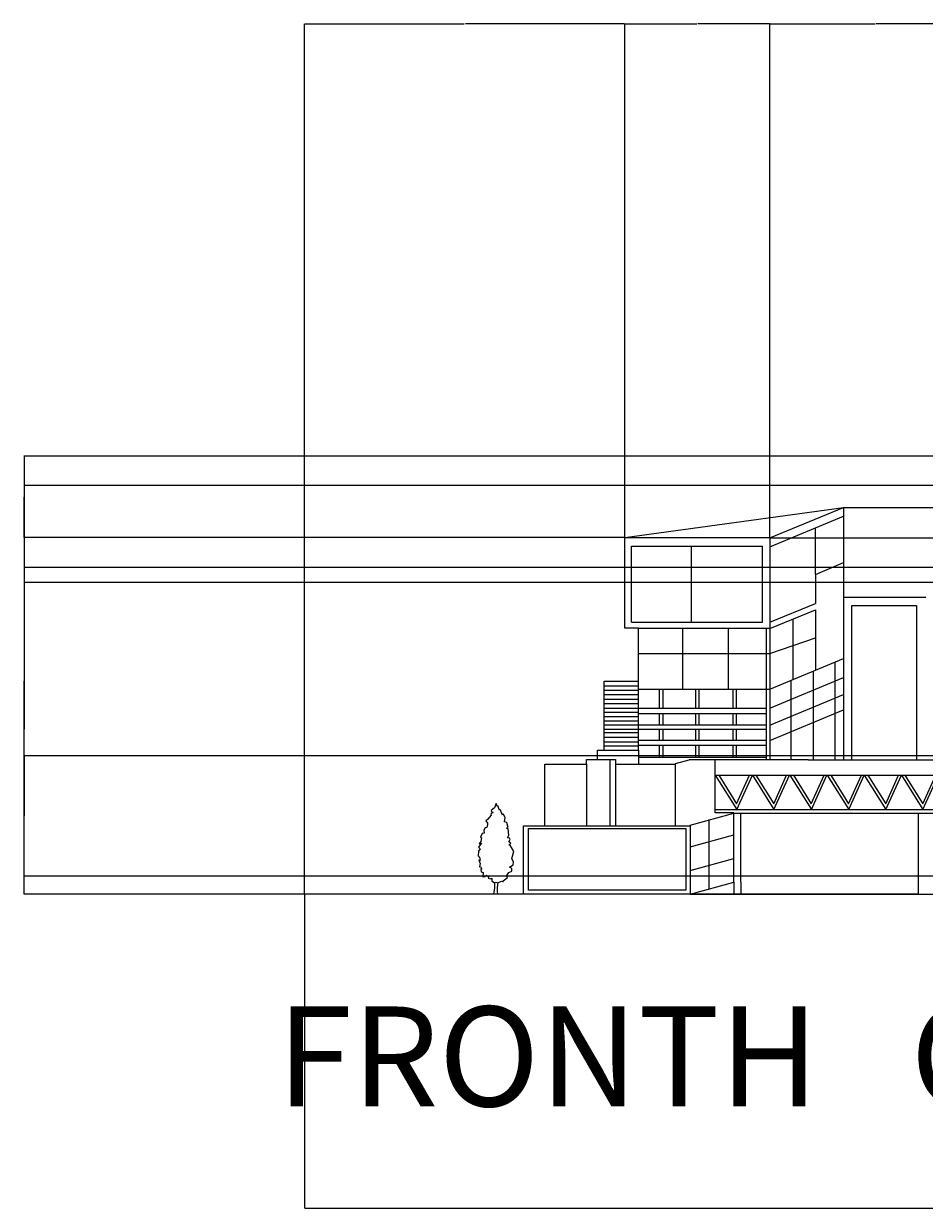
# Model space of a CAD drawing. Units: inches. Extents: x -2248 to 2617, y -128 to 922.
# Tile 1 of 7: x -2248 to -1531, y -128 to 815. Entities that reach past the tile are written whole.
import ezdxf

# ---------------------------------------------------------------- set-up
doc = ezdxf.new("R2010")
doc.units = ezdxf.units.IN
doc.header["$MEASUREMENT"] = 0
for name, color, linetype, lineweight in [('A-ANNO-DIMS', 2, 'Continuous', 18), ('A-ANNO-TEXT', 7, 'Continuous', 25), ('A-ELEV', 7, 'Continuous', 25), ('L-PLNT', 3, 'Continuous', 18)]:
    doc.layers.add(name, color=color, linetype=linetype, lineweight=lineweight)
doc.styles.get("Standard").update_dxf_attribs({"font": 'arial.ttf'})
doc.dimstyles.get("Standard").update_dxf_attribs({"dimtxt": 0.18, "dimasz": 0.18, "dimexe": 0.18, "dimexo": 0.0625, "dimgap": 0.09, "dimtad": 0, "dimtih": 1, "dimtoh": 1, "dimdec": 4, "dimzin": 0, "dimdsep": 46, "dimtxsty": 'Standard', "dimcen": 0.09, "dimadec": 0, "dimazin": 0, "dimtfac": 1, "dimtdec": 4, "dimtofl": 0, "dimtmove": 0, "dimatfit": 3, "dimfxl": 1, "dimtolj": 1, "dimtzin": 0, "dimarcsym": 0})

# ---------------------------------------------------------------- blocks, each defined once
blk = doc.blocks.new('*U3')
blk.add_lwpolyline([(-2.754, 191.699), (-6.78, 182.851), (-13.682, 176.953), (-11.956, 173.266), (-9.656, 172.529), (-14.257, 170.317), (-13.682, 167.368), (-21.733, 157.783), (-25.184, 154.834), (-21.158, 150.41), (-21.733, 147.461), (-22.884, 140.825), (-26.334, 140.087), (-29.21, 134.926), (-28.635, 129.028), (-32.661, 128.291), (-36.111, 120.18), (-34.386, 118.706), (-35.536, 111.333), (-38.987, 106.171), (-34.386, 107.646), (-40.712, 98.798), (-37.261, 95.849), (-40.712, 90.688), (-41.287, 80.366), (-38.412, 78.154), (-36.686, 70.781), (-39.562, 71.518), (-37.261, 64.145), (-38.412, 57.509), (-36.111, 58.247), (-33.236, 52.348), (-35.536, 53.086), (-34.961, 46.45), (-30.36, 44.975), (-31.51, 36.128), (-26.334, 36.865), (-23.459, 39.814), (-18.283, 36.128), (-20.008, 33.178), (-14.832, 31.704), (-11.956, 33.178), (-12.531, 27.28), (-6.205, 22.856), (-3.905, 24.331), (0.121, 22.856), (8.173, 26.543), (11.624, 25.068), (12.199, 27.28), (21.4, 34.653), (19.675, 39.077), (23.701, 44.975), (30.027, 47.924), (30.602, 53.823), (25.426, 56.772), (32.903, 61.196), (34.053, 67.094), (30.602, 75.205), (34.628, 89.951), (26.576, 103.222), (23.701, 103.222), (28.302, 107.646), (23.701, 110.595), (26.576, 115.756), (25.426, 117.968), (20.825, 118.706), (24.276, 124.604), (22.551, 137.876), (19.1, 139.35), (22.551, 140.825), (19.675, 151.884), (14.499, 153.359), (16.224, 162.207), (12.199, 170.317), (10.473, 167.368), (5.872, 179.165), (4.147, 177.69), (0.696, 187.275), (-0.454, 185.8)], close=True)
for points in [[(-6.813, 23.669), (-6.813, 11.669), (-8.627, 0)], [(0.387, 23.669), (-0.576, 13.271), (-0.576, 3.686), (0, 0)]]:
    blk.add_lwpolyline(points)
blk = doc.blocks.new('*D18')
at = {"layer": 'A-ANNO-DIMS', "color": 0, "lineweight": -2, "transparency": 16777216}
for p, q in [((-1769.46, 405.79), (-2247.68, 405.79)), ((-2247.5, 405.61), (-2247.5, 264.12)), ((-2247.5, 122.26), (-2247.5, 263.76)), ((-1850.09, 122.08), (-2247.68, 122.08))]:
    blk.add_line(p, q, dxfattribs=at)
at = {"layer": 'A-ANNO-DIMS', "color": 0, "transparency": 16777216}
for points in [[(-2247.53, 405.61), (-2247.47, 405.61), (-2247.5, 405.79)], [(-2247.53, 122.26), (-2247.47, 122.26), (-2247.5, 122.08)]]:
    blk.add_solid(points, dxfattribs=at)
at = {"layer": 'Defpoints', "color": 0, "transparency": 16777216}
for p in [(-1769.4, 405.79), (-2247.5, 122.08), (-1850.03, 122.08)]:
    blk.add_point(p, dxfattribs=at)
at = {"layer": 'A-ANNO-DIMS', "color": 0, "transparency": 16777216, "insert": (-2247.5, 263.94), "char_height": 0.18, "attachment_point": 5}
blk.add_mtext('\\A1;283.7', dxfattribs=at)
blk = doc.blocks.new('*D19')
at = {"layer": 'A-ANNO-DIMS', "color": 0, "lineweight": -2, "transparency": 16777216}
for p, q in [((-1125.47, 470.63), (-2247.68, 470.63)), ((-2247.5, 470.45), (-2247.5, 438.39)), ((-2247.5, 405.97), (-2247.5, 438.03)), ((-1769.46, 405.79), (-2247.68, 405.79))]:
    blk.add_line(p, q, dxfattribs=at)
at = {"layer": 'A-ANNO-DIMS', "color": 0, "transparency": 16777216}
for points in [[(-2247.53, 470.45), (-2247.47, 470.45), (-2247.5, 470.63)], [(-2247.53, 405.97), (-2247.47, 405.97), (-2247.5, 405.79)]]:
    blk.add_solid(points, dxfattribs=at)
at = {"layer": 'Defpoints', "color": 0, "transparency": 16777216}
for p in [(-1125.41, 470.63), (-2247.5, 405.79), (-1769.4, 405.79)]:
    blk.add_point(p, dxfattribs=at)
at = {"layer": 'A-ANNO-DIMS', "color": 0, "transparency": 16777216, "insert": (-2247.5, 438.21), "char_height": 0.18, "attachment_point": 5}
blk.add_mtext('\\A1;64.83', dxfattribs=at)
blk = doc.blocks.new('*D20')
at = {"layer": 'A-ANNO-DIMS', "color": 0, "lineweight": -2, "transparency": 16777216}
for p, q in [((-1595.32, 429.87), (2616.45, 429.87)), ((2616.27, 429.69), (2616.27, 417.91)), ((2616.27, 405.76), (2616.27, 417.54)), ((-1653.9, 405.58), (2616.45, 405.58))]:
    blk.add_line(p, q, dxfattribs=at)
at = {"layer": 'A-ANNO-DIMS', "color": 0, "transparency": 16777216}
for points in [[(2616.24, 429.69), (2616.3, 429.69), (2616.27, 429.87)], [(2616.24, 405.76), (2616.3, 405.76), (2616.27, 405.58)]]:
    blk.add_solid(points, dxfattribs=at)
at = {"layer": 'Defpoints', "color": 0, "transparency": 16777216}
for p in [(-1595.38, 429.87), (-1653.96, 405.58), (2616.27, 405.58)]:
    blk.add_point(p, dxfattribs=at)
at = {"layer": 'A-ANNO-DIMS', "color": 0, "transparency": 16777216, "insert": (2616.27, 417.72), "char_height": 0.18, "attachment_point": 5}
blk.add_mtext('\\A1;24.3', dxfattribs=at)
blk = doc.blocks.new('*D29')
at = {"layer": 'A-ANNO-DIMS', "color": 0, "lineweight": -2, "transparency": 16777216}
for p, q in [((358.92, 381.97), (-2247.68, 381.97)), ((-2247.5, 381.79), (-2247.5, 259.39)), ((-2247.5, 136.63), (-2247.5, 259.03)), ((392.64, 136.45), (-2247.68, 136.45))]:
    blk.add_line(p, q, dxfattribs=at)
at = {"layer": 'A-ANNO-DIMS', "color": 0, "transparency": 16777216}
for points in [[(-2247.53, 381.79), (-2247.47, 381.79), (-2247.5, 381.97)], [(-2247.53, 136.63), (-2247.47, 136.63), (-2247.5, 136.45)]]:
    blk.add_solid(points, dxfattribs=at)
at = {"layer": 'Defpoints', "color": 0, "transparency": 16777216}
for p in [(358.98, 381.97), (-2247.5, 136.45), (392.7, 136.45)]:
    blk.add_point(p, dxfattribs=at)
at = {"layer": 'A-ANNO-DIMS', "color": 0, "transparency": 16777216, "insert": (-2247.5, 259.21), "char_height": 0.18, "attachment_point": 5}
blk.add_mtext('\\A1;245.5', dxfattribs=at)
blk = doc.blocks.new('*D30')
at = {"layer": 'A-ANNO-DIMS', "color": 0, "lineweight": -2, "transparency": 16777216}
for p, q in [((201.76, 232.05), (-2247.68, 232.05)), ((-2247.5, 231.87), (-2247.5, 184.43)), ((-2247.5, 136.63), (-2247.5, 184.07)), ((210.72, 136.45), (-2247.68, 136.45))]:
    blk.add_line(p, q, dxfattribs=at)
at = {"layer": 'A-ANNO-DIMS', "color": 0, "transparency": 16777216}
for points in [[(-2247.53, 231.87), (-2247.47, 231.87), (-2247.5, 232.05)], [(-2247.53, 136.63), (-2247.47, 136.63), (-2247.5, 136.45)]]:
    blk.add_solid(points, dxfattribs=at)
at = {"layer": 'Defpoints', "color": 0, "transparency": 16777216}
for p in [(201.83, 232.05), (-2247.5, 136.45), (210.78, 136.45)]:
    blk.add_point(p, dxfattribs=at)
at = {"layer": 'A-ANNO-DIMS', "color": 0, "transparency": 16777216, "insert": (-2247.5, 184.25), "char_height": 0.18, "attachment_point": 5}
blk.add_mtext('\\A1;95.6', dxfattribs=at)
blk = doc.blocks.new('*D31')
at = {"layer": 'A-ANNO-DIMS', "color": 0, "lineweight": -2, "transparency": 16777216}
for p, q in [((934.8, 447.18), (-2247.68, 447.18)), ((-2247.5, 447), (-2247.5, 292)), ((-2247.5, 136.63), (-2247.5, 291.63)), ((820.03, 136.45), (-2247.68, 136.45))]:
    blk.add_line(p, q, dxfattribs=at)
at = {"layer": 'A-ANNO-DIMS', "color": 0, "transparency": 16777216}
for points in [[(-2247.53, 447), (-2247.47, 447), (-2247.5, 447.18)], [(-2247.53, 136.63), (-2247.47, 136.63), (-2247.5, 136.45)]]:
    blk.add_solid(points, dxfattribs=at)
at = {"layer": 'Defpoints', "color": 0, "transparency": 16777216}
for p in [(934.86, 447.18), (-2247.5, 136.45), (820.09, 136.45)]:
    blk.add_point(p, dxfattribs=at)
at = {"layer": 'A-ANNO-DIMS', "color": 0, "transparency": 16777216, "insert": (-2247.5, 291.82), "char_height": 0.18, "attachment_point": 5}
blk.add_mtext('\\A1;310.7', dxfattribs=at)
blk = doc.blocks.new('*D32')
at = {"layer": 'A-ANNO-DIMS', "color": 0, "lineweight": -2, "transparency": 16777216}
for p, q in [((-975.29, 369.95), (-2247.68, 369.95)), ((-2247.5, 369.77), (-2247.5, 253.38)), ((-2247.5, 136.63), (-2247.5, 253.02)), ((-1029.87, 136.45), (-2247.68, 136.45))]:
    blk.add_line(p, q, dxfattribs=at)
at = {"layer": 'A-ANNO-DIMS', "color": 0, "transparency": 16777216}
for points in [[(-2247.53, 369.77), (-2247.47, 369.77), (-2247.5, 369.95)], [(-2247.53, 136.63), (-2247.47, 136.63), (-2247.5, 136.45)]]:
    blk.add_solid(points, dxfattribs=at)
at = {"layer": 'Defpoints', "color": 0, "transparency": 16777216}
for p in [(-975.23, 369.95), (-2247.5, 136.45), (-1029.81, 136.45)]:
    blk.add_point(p, dxfattribs=at)
at = {"layer": 'A-ANNO-DIMS', "color": 0, "transparency": 16777216, "insert": (-2247.5, 253.2), "char_height": 0.18, "attachment_point": 5}
blk.add_mtext('\\A1;233.5', dxfattribs=at)
blk = doc.blocks.new('*D33')
at = {"layer": 'A-ANNO-DIMS', "color": 0, "lineweight": -2, "transparency": 16777216}
for p, q in [((2393.02, 136.39), (2393.02, -127.85)), ((-2024.25, 122.02), (-2024.25, -127.85)), ((-2024.07, -127.67), (184.02, -127.67)), ((2392.84, -127.67), (184.75, -127.67))]:
    blk.add_line(p, q, dxfattribs=at)
at = {"layer": 'A-ANNO-DIMS', "color": 0, "transparency": 16777216}
for points in [[(-2024.07, -127.64), (-2024.07, -127.7), (-2024.25, -127.67)], [(2392.84, -127.64), (2392.84, -127.7), (2393.02, -127.67)]]:
    blk.add_solid(points, dxfattribs=at)
at = {"layer": 'Defpoints', "color": 0, "transparency": 16777216}
for p in [(2393.02, 136.45), (-2024.25, 122.08), (2393.02, -127.67)]:
    blk.add_point(p, dxfattribs=at)
at = {"layer": 'A-ANNO-DIMS', "color": 0, "transparency": 16777216, "insert": (184.39, -127.67), "char_height": 0.18, "attachment_point": 5}
blk.add_mtext('\\A1;4417', dxfattribs=at)
blk = doc.blocks.new('*D34')
at = {"layer": 'A-ANNO-DIMS', "color": 0, "lineweight": -2, "transparency": 16777216}
for p, q in [((-2024.25, 122.15), (-2024.25, 814.7)), ((-2024.07, 814.52), (-1897.29, 814.52)), ((-1769.58, 814.52), (-1896.36, 814.52)), ((-1769.4, 405.86), (-1769.4, 814.7))]:
    blk.add_line(p, q, dxfattribs=at)
at = {"layer": 'A-ANNO-DIMS', "color": 0, "transparency": 16777216}
for points in [[(-2024.07, 814.55), (-2024.07, 814.49), (-2024.25, 814.52)], [(-1769.58, 814.55), (-1769.58, 814.49), (-1769.4, 814.52)]]:
    blk.add_solid(points, dxfattribs=at)
at = {"layer": 'Defpoints', "color": 0, "transparency": 16777216}
for p in [(-1769.4, 814.52), (-1769.4, 405.79), (-2024.25, 122.08)]:
    blk.add_point(p, dxfattribs=at)
at = {"layer": 'A-ANNO-DIMS', "color": 0, "transparency": 16777216, "insert": (-1896.83, 814.52), "char_height": 0.18, "attachment_point": 5}
blk.add_mtext('\\A1;254.86', dxfattribs=at)
blk = doc.blocks.new('*D35')
at = {"layer": 'A-ANNO-DIMS', "color": 0, "lineweight": -2, "transparency": 16777216}
for p, q in [((-1769.4, 405.86), (-1769.4, 814.7)), ((-1769.22, 814.52), (-1712.13, 814.52)), ((-1654.14, 814.52), (-1711.22, 814.52)), ((-1653.96, 405.64), (-1653.96, 814.7))]:
    blk.add_line(p, q, dxfattribs=at)
at = {"layer": 'A-ANNO-DIMS', "color": 0, "transparency": 16777216}
for points in [[(-1769.22, 814.55), (-1769.22, 814.49), (-1769.4, 814.52)], [(-1654.14, 814.55), (-1654.14, 814.49), (-1653.96, 814.52)]]:
    blk.add_solid(points, dxfattribs=at)
at = {"layer": 'Defpoints', "color": 0, "transparency": 16777216}
for p in [(-1653.96, 814.52), (-1769.4, 405.79), (-1653.96, 405.58)]:
    blk.add_point(p, dxfattribs=at)
at = {"layer": 'A-ANNO-DIMS', "color": 0, "transparency": 16777216, "insert": (-1711.68, 814.52), "char_height": 0.18, "attachment_point": 5}
blk.add_mtext('\\A1;115.44', dxfattribs=at)
blk = doc.blocks.new('*D36')
at = {"layer": 'A-ANNO-DIMS', "color": 0, "lineweight": -2, "transparency": 16777216}
for p, q in [((-1653.96, 405.64), (-1653.96, 814.7)), ((-1653.78, 814.52), (-1570.34, 814.52)), ((-1485.99, 814.52), (-1569.43, 814.52)), ((-1485.81, 421.23), (-1485.81, 814.7))]:
    blk.add_line(p, q, dxfattribs=at)
at = {"layer": 'A-ANNO-DIMS', "color": 0, "transparency": 16777216}
for points in [[(-1653.78, 814.55), (-1653.78, 814.49), (-1653.96, 814.52)], [(-1485.99, 814.55), (-1485.99, 814.49), (-1485.81, 814.52)]]:
    blk.add_solid(points, dxfattribs=at)
at = {"layer": 'Defpoints', "color": 0, "transparency": 16777216}
for p in [(-1485.81, 814.52), (-1485.81, 421.17), (-1653.96, 405.58)]:
    blk.add_point(p, dxfattribs=at)
at = {"layer": 'A-ANNO-DIMS', "color": 0, "transparency": 16777216, "insert": (-1569.88, 814.52), "char_height": 0.18, "attachment_point": 5}
blk.add_mtext('\\A1;168.15', dxfattribs=at)

msp = doc.modelspace()

# ---------------------------------------------------------------- linework, layer by layer
at = {"layer": 'A-ELEV'}
for p, q in [((-1769.3984, 405.7946), (-1595.3791, 429.8743)), ((-1653.9599, 405.5754), (-1595.3791, 429.8743)), ((-1595.3791, 429.8743), (-1595.3791, 229.0275)), ((-1653.9599, 398.5149), (-1595.3791, 422.8138)), ((-1769.3984, 333.7238), (-1769.3984, 405.7946)), ((-1769.3984, 405.7946), (-1653.9599, 405.7946)), ((-1653.9599, 405.7946), (-1653.9599, 333.7238)), ((-1617.8435, 376.568), (-1617.8435, 413.4957)), ((-1764.0725, 399.1064), (-1659.7808, 399.1064)), ((-1764.0725, 338.4085), (-1764.0725, 399.1064)), ((-1716.3825, 338.4085), (-1716.3825, 399.1064)), ((-1659.7808, 338.4085), (-1659.7808, 399.1064)), ((-1617.8435, 376.568), (-1595.3791, 385.8861)), ((-1617.8435, 376.9364), (-1617.8435, 353.3991)), ((-1595.3791, 358.31), (-1530.0359, 358.31)), ((-1653.9599, 338.4183), (-1617.8435, 353.3991)), ((-1588.8133, 229.0275), (-1588.8133, 351.851)), ((-1588.8133, 351.851), (-1537.2371, 351.851)), ((-1537.2371, 351.851), (-1537.2371, 229.0275)), ((-1653.9599, 333.363), (-1617.8435, 348.3438)), ((-1635.7166, 340.9302), (-1635.7166, 292.7704)), ((-1617.8435, 348.3438), (-1617.8435, 300.184)), ((-1758.5463, 333.7238), (-1769.3984, 333.7238)), ((-1764.0725, 338.4085), (-1659.7808, 338.4085)), ((-1758.5463, 285.2032), (-1758.5463, 333.7238)), ((-1758.5463, 333.7238), (-1653.9599, 333.7238)), ((-1723.333, 285.2032), (-1723.333, 333.7238)), ((-1687.0727, 285.2032), (-1687.0727, 333.7238)), ((-1656.9931, 333.7238), (-1656.9931, 285.2032)), ((-1653.9599, 333.7238), (-1653.9599, 285.2032)), ((-1653.9599, 313.6036), (-1617.8435, 326.1091)), ((-1758.5463, 313.6036), (-1653.9599, 313.6036)), ((-1653.9599, 285.2032), (-1595.3791, 309.5021)), ((-1602.0308, 229.0275), (-1602.0308, 306.743)), ((-1653.9599, 270.1893), (-1595.3791, 294.4881)), ((-1619.2101, 229.0275), (-1619.2101, 299.6172)), ((-1785.7588, 236.7739), (-1785.7588, 291.6603)), ((-1785.7588, 277.1166), (-1785.7588, 291.6603)), ((-1785.7588, 291.6603), (-1758.5463, 291.6603)), ((-1785.7588, 287.8997), (-1758.5463, 287.8997)), ((-1785.7588, 284.3576), (-1758.5463, 284.3576)), ((-1758.5463, 236.7739), (-1758.5463, 285.2032)), ((-1758.5463, 285.2032), (-1653.9599, 285.2032)), ((-1741.8071, 270.1893), (-1741.8071, 285.2032)), ((-1738.8788, 270.1893), (-1738.8788, 285.2032)), ((-1712.9148, 270.1893), (-1712.9148, 285.2032)), ((-1710.1817, 270.1893), (-1710.1817, 285.2032)), ((-1683.2416, 270.1893), (-1683.2416, 285.2032)), ((-1680.7038, 270.1893), (-1680.7038, 285.2032)), ((-1656.9931, 285.2032), (-1656.9931, 229.0275)), ((-1653.9599, 285.2032), (-1653.9599, 229.0275)), ((-1637.1701, 229.0275), (-1637.1701, 292.1675)), ((-1785.7588, 280.9298), (-1758.5463, 280.9298)), ((-1785.7588, 277.2734), (-1758.5463, 277.2734)), ((-1785.7588, 273.8456), (-1758.5463, 273.8456)), ((-1653.9599, 256.5913), (-1595.3791, 280.8902)), ((-1785.7588, 270.1893), (-1758.5463, 270.1893)), ((-1785.7588, 266.8757), (-1758.5463, 266.8757)), ((-1758.5463, 270.1893), (-1656.9931, 270.1893)), ((-1758.5463, 265.8996), (-1656.9931, 265.8996)), ((-1741.8071, 256.5913), (-1741.8071, 265.8996)), ((-1738.8788, 256.5913), (-1738.8788, 265.8996)), ((-1712.9148, 256.5913), (-1712.9148, 265.8996)), ((-1710.1817, 256.5913), (-1710.1817, 265.8996)), ((-1683.2416, 256.5913), (-1683.2416, 265.8996)), ((-1680.7038, 256.5913), (-1680.7038, 265.8996)), ((-1653.9599, 244.364), (-1595.3791, 268.6629)), ((-1785.7588, 263.4479), (-1758.5463, 263.4479)), ((-1785.7588, 260.0201), (-1758.5463, 260.0201)), ((-1785.7588, 256.7827), (-1758.5463, 256.7827)), ((-1656.9931, 256.5913), (-1758.5463, 256.5913)), ((-1785.7588, 253.4691), (-1758.5463, 253.4691)), ((-1785.7588, 250.6126), (-1758.5463, 250.6126)), ((-1785.7588, 247.0705), (-1758.5463, 247.0705)), ((-1758.5463, 253.4206), (-1656.9931, 253.4206)), ((-1741.8071, 244.364), (-1741.8071, 253.4206)), ((-1738.8788, 244.364), (-1738.8788, 253.4206)), ((-1712.9148, 244.364), (-1712.9148, 253.4206)), ((-1710.1817, 244.364), (-1710.1817, 253.4206)), ((-1683.2416, 244.364), (-1683.2416, 253.4206)), ((-1680.7038, 244.364), (-1680.7038, 253.4206)), ((-1791.289, 229.3063), (-1791.289, 236.7739)), ((-1791.289, 236.7739), (-1758.5463, 236.7739)), ((-1785.7588, 243.4142), (-1758.5463, 243.4142)), ((-1785.7588, 240.2149), (-1758.5463, 240.2149)), ((-1656.9931, 244.364), (-1758.5463, 244.364)), ((-1758.5463, 240.7466), (-1656.9931, 240.7466)), ((-1758.5463, 236.7739), (-1758.5463, 225.6317)), ((-1741.8071, 230.9974), (-1741.8071, 240.7466)), ((-1738.8788, 230.9974), (-1738.8788, 240.7466)), ((-1712.9148, 230.9974), (-1712.9148, 240.7466)), ((-1710.1817, 230.9974), (-1710.1817, 240.7466)), ((-1683.2416, 230.9974), (-1683.2416, 240.7466)), ((-1680.7038, 230.9974), (-1680.7038, 240.7466)), ((-1799.8831, 225.6317), (-1799.8831, 229.3063)), ((-1799.8831, 229.3063), (-1776.941, 229.3063)), ((-1781.406, 229.3063), (-1781.406, 176.4052)), ((-1776.941, 229.3063), (-1776.941, 225.6317)), ((-1758.5463, 230.9974), (-1656.9931, 230.9974)), ((-1729.0393, 226.0366), (-1718.1122, 229.0275)), ((-1623.6327, 229.0275), (-1718.1122, 229.0275)), ((-1697.4805, 189.3441), (-1697.4805, 229.0275)), ((-1623.6327, 229.0275), (-1457.3701, 229.0275)), ((-1833.2088, 225.6317), (-1799.8831, 225.6317)), ((-1833.2088, 176.4052), (-1833.2088, 225.6317)), ((-1799.8831, 225.6317), (-1799.8831, 176.4052)), ((-1776.941, 225.6317), (-1729.0393, 225.6317)), ((-1776.941, 225.6317), (-1776.941, 176.4052)), ((-1729.0393, 176.4052), (-1729.0393, 225.6317)), ((-1697.4805, 216.8261), (-1457.3701, 216.8261)), ((-1697.4805, 216.8261), (-1680.3276, 189.3712)), ((-1694.6636, 216.8173), (-1680.4572, 194.0788)), ((-1680.4572, 194.0788), (-1670.1805, 216.8261)), ((-1680.3276, 189.3712), (-1667.9251, 216.8239)), ((-1667.9686, 216.8261), (-1650.8157, 189.3712)), ((-1665.1517, 216.8173), (-1650.9454, 194.0788)), ((-1650.9454, 194.0788), (-1640.6687, 216.8261)), ((-1650.8157, 189.3712), (-1638.4132, 216.8239)), ((-1638.1502, 216.8261), (-1620.9973, 189.3712)), ((-1635.3333, 216.8173), (-1621.1269, 194.0788)), ((-1621.1269, 194.0788), (-1610.8502, 216.8261)), ((-1620.9973, 189.3712), (-1608.5947, 216.8239)), ((-1608.4194, 216.8261), (-1591.2665, 189.3712)), ((-1605.6025, 216.8173), (-1591.3961, 194.0788)), ((-1591.3961, 194.0788), (-1581.1194, 216.8261)), ((-1591.2665, 189.3712), (-1578.864, 216.8239)), ((-1578.8918, 216.8261), (-1561.7389, 189.3712)), ((-1576.0749, 216.8173), (-1561.8686, 194.0788)), ((-1561.8686, 194.0788), (-1551.5919, 216.8261)), ((-1561.7389, 189.3712), (-1549.3364, 216.8239)), ((-1549.3643, 216.8261), (-1532.2114, 189.3712)), ((-1546.5474, 216.8173), (-1532.341, 194.0788)), ((-1532.341, 194.0788), (-1522.0643, 216.8261)), ((-1532.2114, 189.3712), (-1519.8089, 216.8239)), ((-1697.4805, 189.3441), (-1470.1344, 189.3441)), ((-1697.4805, 186.8521), (-1697.4805, 189.3441)), ((-1535.9308, 189.3441), (-1535.908, 189.2941)), ((-1535.908, 189.2941), (-1535.8806, 189.3441)), ((-1717.4681, 177.1095), (-1682.5813, 186.6586)), ((-1702.4754, 181.4068), (-1702.4754, 126.1913)), ((-1682.5813, 186.8521), (-1697.4805, 186.8521)), ((-1682.5813, 131.6366), (-1682.5813, 186.8521)), ((-1682.5813, 186.6586), (-1488.121, 186.6586)), ((-1677.2512, 131.6366), (-1677.2512, 186.8521)), ((-1535.908, 186.6586), (-1535.908, 122.0847)), ((-1850.0291, 122.0847), (-1850.0291, 176.4052)), ((-1850.0291, 176.4052), (-1717.4349, 176.4052)), ((-1846.2091, 174.2719), (-1720.8842, 174.2719)), ((-1846.2091, 125.1542), (-1846.2091, 174.2719)), ((-1720.8842, 174.2719), (-1720.8842, 125.1542)), ((-1717.4681, 177.303), (-1717.4681, 122.0847)), ((-1717.4681, 159.8443), (-1682.5813, 169.3934)), ((-1717.4681, 140.8567), (-1682.5813, 150.4058)), ((-1720.8842, 125.1542), (-1846.2091, 125.1542)), ((-1717.4681, 122.0875), (-1682.5813, 131.6366)), ((-1682.5813, 131.6366), (-1682.5813, 122.0847)), ((-1677.2512, 131.6366), (-1677.2512, 122.0847)), ((-1850.0291, 122.0847), (-2024.254, 122.0847)), ((-1717.4681, 122.0847), (-1850.0291, 122.0847)), ((-1535.908, 122.0847), (-1717.4681, 122.0847)), ((-1717.4681, 122.0847), (-1344.5966, 122.0847))]:
    msp.add_line(p, q, dxfattribs=at)

# ---------------------------------------------------------------- block references
at = {"layer": 'L-PLNT', "xscale": 0.373818396241174, "yscale": 0.373818396241174, "zscale": 0.373818396241174}
msp.add_blockref('*U3', (-1870.7162, 122.4482), dxfattribs=at)

# ---------------------------------------------------------------- texts
at = {"layer": 'A-ANNO-TEXT'}
msp.add_text('FRONTH   ORTHOGONAL    ELEVATION', height=79.456618, dxfattribs=at).set_placement((-2046.3376, -46.7341))

# ---------------------------------------------------------------- dimensions: what is measured, and where the dimension line sits
at = {"layer": 'A-ANNO-DIMS'}
for base, p1, p2, override, picture, middle in [((-1769.3984, 814.5189), (-2024.254, 122.0847), (-1769.3984, 405.7946), {"dimdec": 2, "dimlfac": 1, "dimrnd": 0, "dimzin": 0, "dimdsep": 46, "dimlunit": 2}, '*D34', (-1896.8262, 814.5189)), ((-1653.9599, 814.5189), (-1769.3984, 405.7946), (-1653.9599, 405.5754), {"dimdec": 2, "dimlfac": 1, "dimrnd": 0, "dimzin": 0, "dimdsep": 46, "dimlunit": 2}, '*D35', (-1711.6791, 814.5189)), ((-1485.8077, 814.5189), (-1653.9599, 405.5754), (-1485.8077, 421.1696), {"dimdec": 2, "dimlfac": 1, "dimrnd": 0, "dimzin": 0, "dimdsep": 46, "dimlunit": 2}, '*D36', (-1569.8838, 814.5189)), ((2393.0245, -127.6745), (-2024.254, 122.0847), (2393.0245, 136.4519), {"dimdec": 0, "dimlfac": 1, "dimrnd": 0, "dimzin": 0, "dimdsep": 46, "dimlunit": 2}, '*D33', (184.3853, -127.6745))]:
    dim = msp.add_linear_dim(base=base, p1=p1, p2=p2, dimstyle='Standard', override=override, dxfattribs=at)
    dim.commit()
    dim.dimension.update_dxf_attribs({"geometry": picture, "text_midpoint": middle})
for base, p1, p2, override, picture, middle in [((-2247.504, 405.7946), (-1125.4072, 470.6286), (-1769.3984, 405.7946), {"dimdec": 2, "dimlfac": 1, "dimrnd": 0, "dimzin": 0, "dimdsep": 46, "dimlunit": 2}, '*D19', (-2247.504, 438.2116)), ((-2247.504, 136.4519), (934.8599, 447.1806), (820.0929, 136.4519), {"dimdec": 1, "dimlfac": 1, "dimrnd": 0, "dimzin": 0, "dimdsep": 46, "dimlunit": 2}, '*D31', (-2247.504, 291.8162)), ((2616.2745, 405.5754), (-1595.3791, 429.8743), (-1653.9599, 405.5754), {"dimdec": 1, "dimlfac": 1, "dimrnd": 0, "dimzin": 0, "dimdsep": 46, "dimlunit": 2}, '*D20', (2616.2745, 417.7249)), ((-2247.504, 122.0847), (-1769.3984, 405.7946), (-1850.0291, 122.0847), {"dimdec": 1, "dimlfac": 1, "dimrnd": 0, "dimzin": 0, "dimdsep": 46, "dimlunit": 2}, '*D18', (-2247.504, 263.9397)), ((-2247.504, 136.4519), (358.982, 381.9653), (392.6975, 136.4519), {"dimdec": 1, "dimlfac": 1, "dimrnd": 0, "dimzin": 0, "dimdsep": 46, "dimlunit": 2}, '*D29', (-2247.504, 259.2086)), ((-2247.504, 136.4519), (-975.2258, 369.9469), (-1029.8099, 136.4519), {"dimdec": 1, "dimlfac": 1, "dimrnd": 0, "dimzin": 0, "dimdsep": 46, "dimlunit": 2}, '*D32', (-2247.504, 253.1994)), ((-2247.504, 136.4519), (201.8252, 232.0521), (210.7789, 136.4519), {"dimdec": 1, "dimlfac": 1, "dimrnd": 0, "dimzin": 0, "dimdsep": 46, "dimlunit": 2}, '*D30', (-2247.504, 184.252))]:
    dim = msp.add_linear_dim(base=base, p1=p1, p2=p2, angle=90, dimstyle='Standard', override=override, dxfattribs=at)
    dim.commit()
    dim.dimension.update_dxf_attribs({"geometry": picture, "text_midpoint": middle})

doc.saveas('drawing.dxf')
